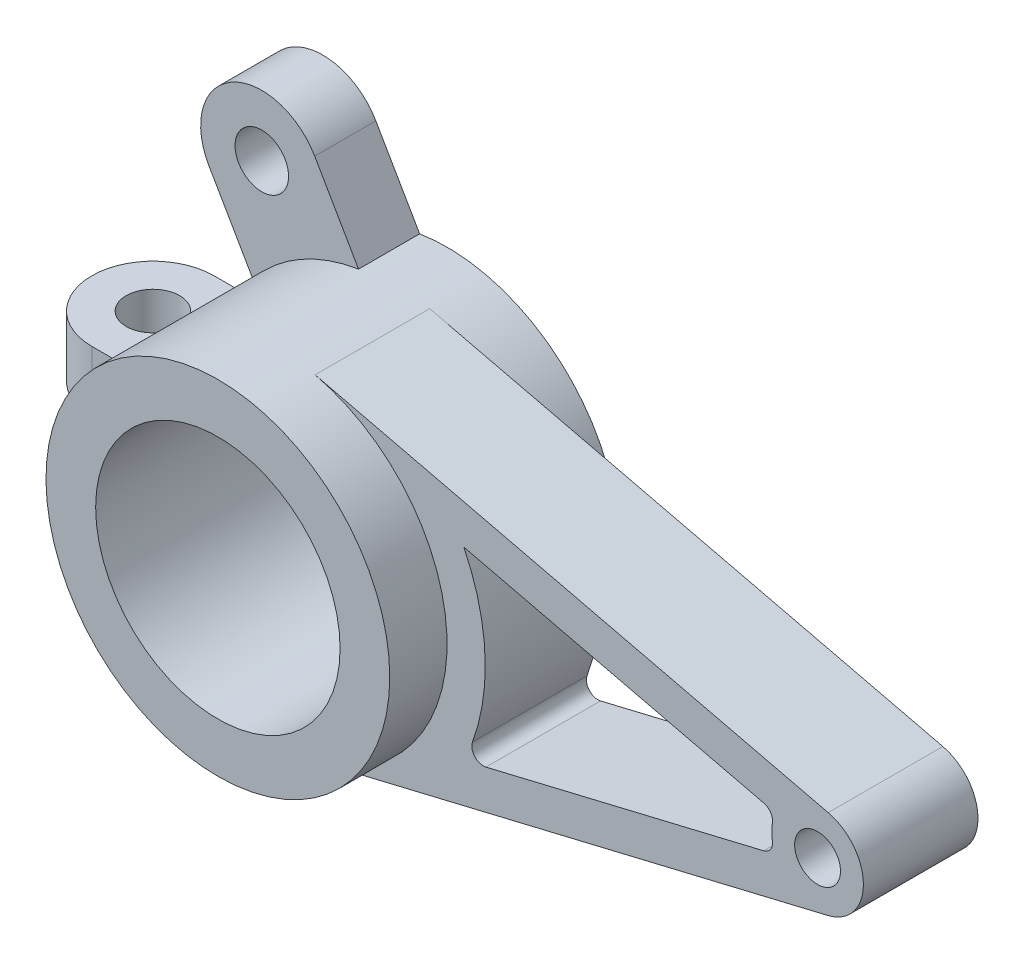
ISO-10303-21;
HEADER;
FILE_DESCRIPTION(('STEP AP214'),'2;1');
FILE_NAME('part.step','',(''),(''),'','','');
FILE_SCHEMA(('AUTOMOTIVE_DESIGN { 1 0 10303 214 1 1 1 1 }'));
ENDSEC;
DATA;
#1=APPLICATION_CONTEXT('core data for automotive mechanical design processes');
#2=APPLICATION_PROTOCOL_DEFINITION('international standard','automotive_design',2000,#1);
#3=PRODUCT_CONTEXT('',#1,'mechanical');
#4=PRODUCT('Part','Part','',(#3));
#5=PRODUCT_RELATED_PRODUCT_CATEGORY('part','',(#4));
#6=PRODUCT_DEFINITION_FORMATION('','',#4);
#7=PRODUCT_DEFINITION_CONTEXT('part definition',#1,'design');
#8=PRODUCT_DEFINITION('design','',#6,#7);
#9=PRODUCT_DEFINITION_SHAPE('','',#8);
#10=(LENGTH_UNIT() NAMED_UNIT(*) SI_UNIT(.MILLI.,.METRE.));
#11=(NAMED_UNIT(*) PLANE_ANGLE_UNIT() SI_UNIT($,.RADIAN.));
#12=(NAMED_UNIT(*) SI_UNIT($,.STERADIAN.) SOLID_ANGLE_UNIT());
#13=UNCERTAINTY_MEASURE_WITH_UNIT(LENGTH_MEASURE(1.E-05),#10,'distance_accuracy_value','');
#14=(GEOMETRIC_REPRESENTATION_CONTEXT(3) GLOBAL_UNCERTAINTY_ASSIGNED_CONTEXT((#13)) GLOBAL_UNIT_ASSIGNED_CONTEXT((#10,
#11,#12)) REPRESENTATION_CONTEXT('',''));
#15=CARTESIAN_POINT('',(0.,0.,0.));
#16=DIRECTION('',(0.,0.,1.));
#17=DIRECTION('',(1.,0.,0.));
#18=AXIS2_PLACEMENT_3D('',#15,#16,#17);
#19=CARTESIAN_POINT('',(0.,0.,60.));
#20=DIRECTION('',(0.,0.,-1.));
#21=DIRECTION('',(-1.,0.,0.));
#22=AXIS2_PLACEMENT_3D('',#19,#20,#21);
#23=CYLINDRICAL_SURFACE('',#22,45.);
#24=DIRECTION('',(0.,0.,-1.));
#25=VECTOR('',#24,1.);
#26=CARTESIAN_POINT('',(10.4577464788732,-43.7679738916895,45.));
#27=LINE('',#26,#25);
#28=CARTESIAN_POINT('',(10.4577464788732,-43.7679738916895,45.));
#29=VERTEX_POINT('',#28);
#30=CARTESIAN_POINT('',(10.4577464788732,-43.7679738916895,15.));
#31=VERTEX_POINT('',#30);
#32=EDGE_CURVE('E369',#29,#31,#27,.T.);
#33=ORIENTED_EDGE('',*,*,#32,.F.);
#34=CARTESIAN_POINT('',(0.,0.,45.));
#35=DIRECTION('',(0.,0.,1.));
#36=DIRECTION('',(1.,0.,0.));
#37=AXIS2_PLACEMENT_3D('',#34,#35,#36);
#38=CIRCLE('',#37,45.);
#39=CARTESIAN_POINT('',(10.4577464788732,43.7679738916895,45.));
#40=VERTEX_POINT('',#39);
#41=EDGE_CURVE('E332',#29,#40,#38,.T.);
#42=ORIENTED_EDGE('',*,*,#41,.T.);
#43=DIRECTION('',(0.,0.,-1.));
#44=VECTOR('',#43,1.);
#45=CARTESIAN_POINT('',(10.4577464788732,43.7679738916895,45.));
#46=LINE('',#45,#44);
#47=CARTESIAN_POINT('',(10.4577464788732,43.7679738916895,15.));
#48=VERTEX_POINT('',#47);
#49=EDGE_CURVE('E373',#40,#48,#46,.T.);
#50=ORIENTED_EDGE('',*,*,#49,.T.);
#51=CARTESIAN_POINT('',(0.,0.,15.));
#52=DIRECTION('',(0.,0.,1.));
#53=DIRECTION('',(1.,0.,0.));
#54=AXIS2_PLACEMENT_3D('',#51,#52,#53);
#55=CIRCLE('',#54,45.);
#56=EDGE_CURVE('E306',#31,#48,#55,.T.);
#57=ORIENTED_EDGE('',*,*,#56,.F.);
#58=EDGE_LOOP('',(#33,#42,#50,#57));
#59=FACE_BOUND('',#58,.T.);
#60=CARTESIAN_POINT('',(0.,0.,60.));
#61=DIRECTION('',(0.,0.,1.));
#62=DIRECTION('',(1.,0.,0.));
#63=AXIS2_PLACEMENT_3D('',#60,#61,#62);
#64=CIRCLE('',#63,45.);
#65=CARTESIAN_POINT('',(45.,0.,60.));
#66=VERTEX_POINT('',#65);
#67=EDGE_CURVE('E49',#66,#66,#64,.T.);
#68=ORIENTED_EDGE('',*,*,#67,.F.);
#69=EDGE_LOOP('',(#68));
#70=FACE_BOUND('',#69,.T.);
#71=CARTESIAN_POINT('',(0.,0.,0.));
#72=DIRECTION('',(0.,0.,1.));
#73=DIRECTION('',(1.,0.,0.));
#74=AXIS2_PLACEMENT_3D('',#71,#72,#73);
#75=CIRCLE('',#74,45.);
#76=CARTESIAN_POINT('',(-34.8861473053641,28.4245796132227,0.));
#77=VERTEX_POINT('',#76);
#78=CARTESIAN_POINT('',(-44.2831796509691,8.,0.));
#79=VERTEX_POINT('',#78);
#80=EDGE_CURVE('E405',#77,#79,#75,.T.);
#81=ORIENTED_EDGE('',*,*,#80,.T.);
#82=DIRECTION('',(0.,0.,-1.));
#83=VECTOR('',#82,1.);
#84=CARTESIAN_POINT('',(-44.2831796509691,8.,60.));
#85=LINE('',#84,#83);
#86=CARTESIAN_POINT('',(-44.2831796509691,8.,32.));
#87=VERTEX_POINT('',#86);
#88=EDGE_CURVE('E60',#79,#87,#85,.F.);
#89=ORIENTED_EDGE('',*,*,#88,.T.);
#90=CARTESIAN_POINT('',(0.,0.,32.));
#91=DIRECTION('',(0.,0.,-1.));
#92=DIRECTION('',(-1.,0.,0.));
#93=AXIS2_PLACEMENT_3D('',#90,#91,#92);
#94=CIRCLE('',#93,45.);
#95=CARTESIAN_POINT('',(-44.2831796509691,-8.,32.));
#96=VERTEX_POINT('',#95);
#97=EDGE_CURVE('E11',#96,#87,#94,.T.);
#98=ORIENTED_EDGE('',*,*,#97,.F.);
#99=DIRECTION('',(0.,0.,-1.));
#100=VECTOR('',#99,1.);
#101=CARTESIAN_POINT('',(-44.2831796509691,-8.,60.));
#102=LINE('',#101,#100);
#103=CARTESIAN_POINT('',(-44.2831796509691,-8.,0.));
#104=VERTEX_POINT('',#103);
#105=EDGE_CURVE('E65',#104,#96,#102,.F.);
#106=ORIENTED_EDGE('',*,*,#105,.F.);
#107=CARTESIAN_POINT('',(-35.9271712475847,-27.0968331387032,0.));
#108=VERTEX_POINT('',#107);
#109=EDGE_CURVE('E401',#104,#108,#75,.T.);
#110=ORIENTED_EDGE('',*,*,#109,.T.);
#111=DIRECTION('',(0.,0.,-1.));
#112=VECTOR('',#111,1.);
#113=CARTESIAN_POINT('',(-35.9271712475847,-27.0968331387032,16.));
#114=LINE('',#113,#112);
#115=CARTESIAN_POINT('',(-35.9271712475847,-27.0968331387032,16.));
#116=VERTEX_POINT('',#115);
#117=EDGE_CURVE('E263',#116,#108,#114,.T.);
#118=ORIENTED_EDGE('',*,*,#117,.F.);
#119=CARTESIAN_POINT('',(0.,0.,16.));
#120=DIRECTION('',(0.,0.,1.));
#121=DIRECTION('',(1.,0.,0.));
#122=AXIS2_PLACEMENT_3D('',#119,#120,#121);
#123=CIRCLE('',#122,45.);
#124=CARTESIAN_POINT('',(-8.83362462507804,-44.1244498660688,16.));
#125=VERTEX_POINT('',#124);
#126=EDGE_CURVE('E234',#116,#125,#123,.T.);
#127=ORIENTED_EDGE('',*,*,#126,.T.);
#128=DIRECTION('',(0.,0.,-1.));
#129=VECTOR('',#128,1.);
#130=CARTESIAN_POINT('',(-8.83362462507804,-44.1244498660688,16.));
#131=LINE('',#130,#129);
#132=CARTESIAN_POINT('',(-8.83362462507804,-44.1244498660688,0.));
#133=VERTEX_POINT('',#132);
#134=EDGE_CURVE('E250',#125,#133,#131,.T.);
#135=ORIENTED_EDGE('',*,*,#134,.T.);
#136=CARTESIAN_POINT('',(-7.17333438426207,44.4245796132227,0.));
#137=VERTEX_POINT('',#136);
#138=EDGE_CURVE('E397',#133,#137,#75,.T.);
#139=ORIENTED_EDGE('',*,*,#138,.T.);
#140=DIRECTION('',(0.,0.,-1.));
#141=VECTOR('',#140,1.);
#142=CARTESIAN_POINT('',(-7.17333438426207,44.4245796132227,16.));
#143=LINE('',#142,#141);
#144=CARTESIAN_POINT('',(-7.17333438426207,44.4245796132227,16.));
#145=VERTEX_POINT('',#144);
#146=EDGE_CURVE('E296',#145,#137,#143,.T.);
#147=ORIENTED_EDGE('',*,*,#146,.F.);
#148=CARTESIAN_POINT('',(0.,0.,16.));
#149=DIRECTION('',(0.,0.,-1.));
#150=DIRECTION('',(1.,0.,0.));
#151=AXIS2_PLACEMENT_3D('',#148,#149,#150);
#152=CIRCLE('',#151,45.);
#153=CARTESIAN_POINT('',(-34.8861473053641,28.4245796132227,16.));
#154=VERTEX_POINT('',#153);
#155=EDGE_CURVE('E274',#154,#145,#152,.T.);
#156=ORIENTED_EDGE('',*,*,#155,.F.);
#157=DIRECTION('',(0.,0.,-1.));
#158=VECTOR('',#157,1.);
#159=CARTESIAN_POINT('',(-34.8861473053641,28.4245796132227,16.));
#160=LINE('',#159,#158);
#161=EDGE_CURVE('E285',#154,#77,#160,.T.);
#162=ORIENTED_EDGE('',*,*,#161,.T.);
#163=EDGE_LOOP('',(#81,#89,#98,#106,#110,#118,#127,#135,#139,#147,#156,#162));
#164=FACE_BOUND('',#163,.T.);
#165=ADVANCED_FACE('F43',(#59,#70,#164),#23,.T.);
#166=CARTESIAN_POINT('',(0.,0.,60.));
#167=DIRECTION('',(0.,0.,1.));
#168=DIRECTION('',(1.,0.,0.));
#169=AXIS2_PLACEMENT_3D('',#166,#167,#168);
#170=PLANE('',#169);
#171=ORIENTED_EDGE('',*,*,#67,.T.);
#172=EDGE_LOOP('',(#171));
#173=FACE_BOUND('',#172,.T.);
#174=CARTESIAN_POINT('',(0.,0.,60.));
#175=DIRECTION('',(0.,0.,1.));
#176=DIRECTION('',(1.,0.,0.));
#177=AXIS2_PLACEMENT_3D('',#174,#175,#176);
#178=CIRCLE('',#177,32.);
#179=CARTESIAN_POINT('',(32.,0.,60.));
#180=VERTEX_POINT('',#179);
#181=EDGE_CURVE('E395',#180,#180,#178,.T.);
#182=ORIENTED_EDGE('',*,*,#181,.F.);
#183=EDGE_LOOP('',(#182));
#184=FACE_BOUND('',#183,.T.);
#185=ADVANCED_FACE('F432',(#173,#184),#170,.T.);
#186=CARTESIAN_POINT('',(0.,0.,0.));
#187=DIRECTION('',(0.,0.,1.));
#188=DIRECTION('',(1.,0.,0.));
#189=AXIS2_PLACEMENT_3D('',#186,#187,#188);
#190=PLANE('',#189);
#191=ORIENTED_EDGE('',*,*,#109,.F.);
#192=DIRECTION('',(-1.,0.,0.));
#193=VECTOR('',#192,1.);
#194=CARTESIAN_POINT('',(-61.,-8.,0.));
#195=LINE('',#194,#193);
#196=CARTESIAN_POINT('',(-61.,-8.,0.));
#197=VERTEX_POINT('',#196);
#198=EDGE_CURVE('E208',#104,#197,#195,.T.);
#199=ORIENTED_EDGE('',*,*,#198,.T.);
#200=DIRECTION('',(0.,-1.,0.));
#201=VECTOR('',#200,1.);
#202=CARTESIAN_POINT('',(-61.,8.,0.));
#203=LINE('',#202,#201);
#204=CARTESIAN_POINT('',(-61.,8.,0.));
#205=VERTEX_POINT('',#204);
#206=EDGE_CURVE('E207',#205,#197,#203,.T.);
#207=ORIENTED_EDGE('',*,*,#206,.F.);
#208=DIRECTION('',(-1.,0.,0.));
#209=VECTOR('',#208,1.);
#210=CARTESIAN_POINT('',(-45.,8.,0.));
#211=LINE('',#210,#209);
#212=EDGE_CURVE('E191',#79,#205,#211,.T.);
#213=ORIENTED_EDGE('',*,*,#212,.F.);
#214=ORIENTED_EDGE('',*,*,#80,.F.);
#215=DIRECTION('',(0.5,-0.866025403784439,0.));
#216=VECTOR('',#215,1.);
#217=CARTESIAN_POINT('',(-34.8861473053641,28.4245796132227,0.));
#218=LINE('',#217,#216);
#219=CARTESIAN_POINT('',(-46.356406460551,48.2916512459885,0.));
#220=VERTEX_POINT('',#219);
#221=EDGE_CURVE('E279',#220,#77,#218,.T.);
#222=ORIENTED_EDGE('',*,*,#221,.F.);
#223=CARTESIAN_POINT('',(-32.5000000000001,56.2916512459885,0.));
#224=DIRECTION('',(0.,0.,1.));
#225=DIRECTION('',(1.,0.,0.));
#226=AXIS2_PLACEMENT_3D('',#223,#224,#225);
#227=CIRCLE('',#226,16.);
#228=CARTESIAN_POINT('',(-18.6435935394491,64.2916512459885,0.));
#229=VERTEX_POINT('',#228);
#230=EDGE_CURVE('E289',#229,#220,#227,.T.);
#231=ORIENTED_EDGE('',*,*,#230,.F.);
#232=DIRECTION('',(-0.5,0.866025403784439,0.));
#233=VECTOR('',#232,1.);
#234=CARTESIAN_POINT('',(-7.17333438426207,44.4245796132227,0.));
#235=LINE('',#234,#233);
#236=EDGE_CURVE('E272',#137,#229,#235,.T.);
#237=ORIENTED_EDGE('',*,*,#236,.F.);
#238=ORIENTED_EDGE('',*,*,#138,.F.);
#239=DIRECTION('',(-0.532113022730173,-0.846673331953333,0.));
#240=VECTOR('',#239,1.);
#241=CARTESIAN_POINT('',(13.5467733112533,-8.51380836368278,0.));
#242=LINE('',#241,#240);
#243=CARTESIAN_POINT('',(-21.0405731662079,-63.5475749406494,0.));
#244=VERTEX_POINT('',#243);
#245=EDGE_CURVE('E255',#133,#244,#242,.T.);
#246=ORIENTED_EDGE('',*,*,#245,.T.);
#247=CARTESIAN_POINT('',(-34.5873464774612,-55.0337665769666,0.));
#248=DIRECTION('',(0.,0.,1.));
#249=DIRECTION('',(1.,0.,0.));
#250=AXIS2_PLACEMENT_3D('',#247,#248,#249);
#251=CIRCLE('',#250,16.);
#252=CARTESIAN_POINT('',(-48.1341197887146,-46.5199582132839,0.));
#253=VERTEX_POINT('',#252);
#254=EDGE_CURVE('E248',#253,#244,#251,.T.);
#255=ORIENTED_EDGE('',*,*,#254,.F.);
#256=DIRECTION('',(-0.532113022730173,-0.846673331953333,0.));
#257=VECTOR('',#256,1.);
#258=CARTESIAN_POINT('',(-13.5467733112533,8.51380836368277,0.));
#259=LINE('',#258,#257);
#260=EDGE_CURVE('E231',#108,#253,#259,.T.);
#261=ORIENTED_EDGE('',*,*,#260,.F.);
#262=EDGE_LOOP('',(#191,#199,#207,#213,#214,#222,#231,#237,#238,#246,#255,#261));
#263=FACE_BOUND('',#262,.T.);
#264=CARTESIAN_POINT('',(0.,0.,0.));
#265=DIRECTION('',(0.,0.,1.));
#266=DIRECTION('',(1.,0.,0.));
#267=AXIS2_PLACEMENT_3D('',#264,#265,#266);
#268=CIRCLE('',#267,32.);
#269=CARTESIAN_POINT('',(32.,0.,0.));
#270=VERTEX_POINT('',#269);
#271=EDGE_CURVE('E382',#270,#270,#268,.T.);
#272=ORIENTED_EDGE('',*,*,#271,.T.);
#273=EDGE_LOOP('',(#272));
#274=FACE_BOUND('',#273,.T.);
#275=CARTESIAN_POINT('',(-32.5000000000001,56.2916512459885,0.));
#276=DIRECTION('',(0.,0.,1.));
#277=DIRECTION('',(1.,0.,0.));
#278=AXIS2_PLACEMENT_3D('',#275,#276,#277);
#279=CIRCLE('',#278,7.);
#280=CARTESIAN_POINT('',(-25.5000000000001,56.2916512459885,0.));
#281=VERTEX_POINT('',#280);
#282=EDGE_CURVE('E269',#281,#281,#279,.T.);
#283=ORIENTED_EDGE('',*,*,#282,.T.);
#284=EDGE_LOOP('',(#283));
#285=FACE_BOUND('',#284,.T.);
#286=CARTESIAN_POINT('',(-34.5873464774612,-55.0337665769666,0.));
#287=DIRECTION('',(0.,0.,1.));
#288=DIRECTION('',(1.,0.,0.));
#289=AXIS2_PLACEMENT_3D('',#286,#287,#288);
#290=CIRCLE('',#289,7.);
#291=CARTESIAN_POINT('',(-27.5873464774612,-55.0337665769666,0.));
#292=VERTEX_POINT('',#291);
#293=EDGE_CURVE('E240',#292,#292,#290,.T.);
#294=ORIENTED_EDGE('',*,*,#293,.T.);
#295=EDGE_LOOP('',(#294));
#296=FACE_BOUND('',#295,.T.);
#297=ADVANCED_FACE('F210',(#263,#274,#285,#296),#190,.F.);
#298=CARTESIAN_POINT('',(0.,0.,60.));
#299=DIRECTION('',(0.,0.,-1.));
#300=DIRECTION('',(-1.,0.,0.));
#301=AXIS2_PLACEMENT_3D('',#298,#299,#300);
#302=CYLINDRICAL_SURFACE('',#301,32.);
#303=ORIENTED_EDGE('',*,*,#181,.T.);
#304=EDGE_LOOP('',(#303));
#305=FACE_BOUND('',#304,.T.);
#306=ORIENTED_EDGE('',*,*,#271,.F.);
#307=EDGE_LOOP('',(#306));
#308=FACE_BOUND('',#307,.T.);
#309=ADVANCED_FACE('F446',(#305,#308),#302,.F.);
#310=CARTESIAN_POINT('',(10.4577464788732,-43.7679738916895,45.));
#311=DIRECTION('',(-0.232394366197183,0.972621642037545,0.));
#312=DIRECTION('',(-0.972621642037545,-0.232394366197183,0.));
#313=AXIS2_PLACEMENT_3D('',#310,#311,#312);
#314=PLANE('',#313);
#315=DIRECTION('',(0.972621642037545,0.232394366197183,0.));
#316=VECTOR('',#315,1.);
#317=CARTESIAN_POINT('',(10.4577464788732,-43.7679738916895,15.));
#318=LINE('',#317,#316);
#319=CARTESIAN_POINT('',(144.788732394366,-11.6714597044506,15.));
#320=VERTEX_POINT('',#319);
#321=EDGE_CURVE('E360',#31,#320,#318,.T.);
#322=ORIENTED_EDGE('',*,*,#321,.T.);
#323=DIRECTION('',(0.,0.,-1.));
#324=VECTOR('',#323,1.);
#325=CARTESIAN_POINT('',(144.788732394366,-11.6714597044506,45.));
#326=LINE('',#325,#324);
#327=CARTESIAN_POINT('',(144.788732394366,-11.6714597044506,45.));
#328=VERTEX_POINT('',#327);
#329=EDGE_CURVE('E377',#328,#320,#326,.T.);
#330=ORIENTED_EDGE('',*,*,#329,.F.);
#331=DIRECTION('',(0.972621642037545,0.232394366197183,0.));
#332=VECTOR('',#331,1.);
#333=CARTESIAN_POINT('',(10.4577464788732,-43.7679738916895,45.));
#334=LINE('',#333,#332);
#335=EDGE_CURVE('E323',#29,#328,#334,.T.);
#336=ORIENTED_EDGE('',*,*,#335,.F.);
#337=ORIENTED_EDGE('',*,*,#32,.T.);
#338=EDGE_LOOP('',(#322,#330,#336,#337));
#339=FACE_BOUND('',#338,.T.);
#340=ADVANCED_FACE('F455',(#339),#314,.F.);
#341=CARTESIAN_POINT('',(142.,0.,45.));
#342=DIRECTION('',(0.,0.,-1.));
#343=DIRECTION('',(-1.,0.,0.));
#344=AXIS2_PLACEMENT_3D('',#341,#342,#343);
#345=CYLINDRICAL_SURFACE('',#344,12.);
#346=CARTESIAN_POINT('',(142.,0.,15.));
#347=DIRECTION('',(0.,0.,1.));
#348=DIRECTION('',(1.,0.,0.));
#349=AXIS2_PLACEMENT_3D('',#346,#347,#348);
#350=CIRCLE('',#349,12.);
#351=CARTESIAN_POINT('',(144.788732394366,11.6714597044505,15.));
#352=VERTEX_POINT('',#351);
#353=EDGE_CURVE('E365',#320,#352,#350,.T.);
#354=ORIENTED_EDGE('',*,*,#353,.T.);
#355=DIRECTION('',(0.,0.,-1.));
#356=VECTOR('',#355,1.);
#357=CARTESIAN_POINT('',(144.788732394366,11.6714597044505,45.));
#358=LINE('',#357,#356);
#359=CARTESIAN_POINT('',(144.788732394366,11.6714597044505,45.));
#360=VERTEX_POINT('',#359);
#361=EDGE_CURVE('E376',#360,#352,#358,.T.);
#362=ORIENTED_EDGE('',*,*,#361,.F.);
#363=CARTESIAN_POINT('',(142.,0.,45.));
#364=DIRECTION('',(0.,0.,1.));
#365=DIRECTION('',(1.,0.,0.));
#366=AXIS2_PLACEMENT_3D('',#363,#364,#365);
#367=CIRCLE('',#366,12.);
#368=EDGE_CURVE('E329',#328,#360,#367,.T.);
#369=ORIENTED_EDGE('',*,*,#368,.F.);
#370=ORIENTED_EDGE('',*,*,#329,.T.);
#371=EDGE_LOOP('',(#354,#362,#369,#370));
#372=FACE_BOUND('',#371,.T.);
#373=ADVANCED_FACE('F506',(#372),#345,.T.);
#374=CARTESIAN_POINT('',(10.4577464788732,43.7679738916895,45.));
#375=DIRECTION('',(0.232394366197183,0.972621642037545,0.));
#376=DIRECTION('',(-0.972621642037545,0.232394366197183,0.));
#377=AXIS2_PLACEMENT_3D('',#374,#375,#376);
#378=PLANE('',#377);
#379=DIRECTION('',(0.972621642037545,-0.232394366197183,0.));
#380=VECTOR('',#379,1.);
#381=CARTESIAN_POINT('',(10.4577464788732,43.7679738916895,15.));
#382=LINE('',#381,#380);
#383=EDGE_CURVE('E362',#48,#352,#382,.T.);
#384=ORIENTED_EDGE('',*,*,#383,.F.);
#385=ORIENTED_EDGE('',*,*,#49,.F.);
#386=DIRECTION('',(0.972621642037545,-0.232394366197183,0.));
#387=VECTOR('',#386,1.);
#388=CARTESIAN_POINT('',(10.4577464788732,43.7679738916895,45.));
#389=LINE('',#388,#387);
#390=EDGE_CURVE('E330',#40,#360,#389,.T.);
#391=ORIENTED_EDGE('',*,*,#390,.T.);
#392=ORIENTED_EDGE('',*,*,#361,.T.);
#393=EDGE_LOOP('',(#384,#385,#391,#392));
#394=FACE_BOUND('',#393,.T.);
#395=ADVANCED_FACE('F505',(#394),#378,.T.);
#396=CARTESIAN_POINT('',(127.210737827939,-2.50553874566784,45.));
#397=DIRECTION('',(0.,0.,-1.));
#398=DIRECTION('',(-1.,0.,0.));
#399=AXIS2_PLACEMENT_3D('',#396,#397,#398);
#400=CYLINDRICAL_SURFACE('',#399,2.99999999999999);
#401=CARTESIAN_POINT('',(127.210737827939,-2.50553874566784,15.));
#402=DIRECTION('',(0.,0.,1.));
#403=DIRECTION('',(1.,0.,0.));
#404=AXIS2_PLACEMENT_3D('',#401,#402,#403);
#405=CIRCLE('',#404,2.99999999999999);
#406=CARTESIAN_POINT('',(127.90792092653,-5.42340367178045,15.));
#407=VERTEX_POINT('',#406);
#408=CARTESIAN_POINT('',(130.168590262351,-2.00443099653427,15.));
#409=VERTEX_POINT('',#408);
#410=EDGE_CURVE('E336',#407,#409,#405,.T.);
#411=ORIENTED_EDGE('',*,*,#410,.F.);
#412=DIRECTION('',(0.,0.,-1.));
#413=VECTOR('',#412,1.);
#414=CARTESIAN_POINT('',(127.90792092653,-5.42340367178045,45.));
#415=LINE('',#414,#413);
#416=CARTESIAN_POINT('',(127.90792092653,-5.42340367178045,45.));
#417=VERTEX_POINT('',#416);
#418=EDGE_CURVE('E372',#417,#407,#415,.T.);
#419=ORIENTED_EDGE('',*,*,#418,.F.);
#420=CARTESIAN_POINT('',(127.210737827939,-2.50553874566784,45.));
#421=DIRECTION('',(0.,0.,1.));
#422=DIRECTION('',(1.,0.,0.));
#423=AXIS2_PLACEMENT_3D('',#420,#421,#422);
#424=CIRCLE('',#423,2.99999999999999);
#425=CARTESIAN_POINT('',(130.168590262351,-2.00443099653427,45.));
#426=VERTEX_POINT('',#425);
#427=EDGE_CURVE('E304',#417,#426,#424,.T.);
#428=ORIENTED_EDGE('',*,*,#427,.T.);
#429=DIRECTION('',(0.,0.,-1.));
#430=VECTOR('',#429,1.);
#431=CARTESIAN_POINT('',(130.168590262351,-2.00443099653427,45.));
#432=LINE('',#431,#430);
#433=EDGE_CURVE('E331',#426,#409,#432,.T.);
#434=ORIENTED_EDGE('',*,*,#433,.T.);
#435=EDGE_LOOP('',(#411,#419,#428,#434));
#436=FACE_BOUND('',#435,.T.);
#437=ADVANCED_FACE('F504',(#436),#400,.F.);
#438=CARTESIAN_POINT('',(8.13380281690141,-34.0417574713141,45.));
#439=DIRECTION('',(-0.232394366197183,0.972621642037545,0.));
#440=DIRECTION('',(-0.972621642037545,-0.232394366197183,0.));
#441=AXIS2_PLACEMENT_3D('',#438,#439,#440);
#442=PLANE('',#441);
#443=DIRECTION('',(0.972621642037545,0.232394366197183,0.));
#444=VECTOR('',#443,1.);
#445=CARTESIAN_POINT('',(8.13380281690141,-34.0417574713141,15.));
#446=LINE('',#445,#444);
#447=CARTESIAN_POINT('',(55.1829610349817,-22.800017794109,15.));
#448=VERTEX_POINT('',#447);
#449=EDGE_CURVE('E342',#448,#407,#446,.T.);
#450=ORIENTED_EDGE('',*,*,#449,.F.);
#451=DIRECTION('',(0.,0.,-1.));
#452=VECTOR('',#451,1.);
#453=CARTESIAN_POINT('',(55.1829610349817,-22.800017794109,45.));
#454=LINE('',#453,#452);
#455=CARTESIAN_POINT('',(55.1829610349817,-22.800017794109,45.));
#456=VERTEX_POINT('',#455);
#457=EDGE_CURVE('E392',#456,#448,#454,.T.);
#458=ORIENTED_EDGE('',*,*,#457,.F.);
#459=DIRECTION('',(0.972621642037545,0.232394366197183,0.));
#460=VECTOR('',#459,1.);
#461=CARTESIAN_POINT('',(8.13380281690141,-34.0417574713141,45.));
#462=LINE('',#461,#460);
#463=EDGE_CURVE('E307',#456,#417,#462,.T.);
#464=ORIENTED_EDGE('',*,*,#463,.T.);
#465=ORIENTED_EDGE('',*,*,#418,.T.);
#466=EDGE_LOOP('',(#450,#458,#464,#465));
#467=FACE_BOUND('',#466,.T.);
#468=ADVANCED_FACE('F531',(#467),#442,.T.);
#469=CARTESIAN_POINT('',(54.4857779363902,-19.8821528679964,45.));
#470=DIRECTION('',(0.,0.,-1.));
#471=DIRECTION('',(-1.,0.,0.));
#472=AXIS2_PLACEMENT_3D('',#469,#470,#471);
#473=CYLINDRICAL_SURFACE('',#472,3.00000000000001);
#474=CARTESIAN_POINT('',(54.4857779363902,-19.8821528679964,15.));
#475=DIRECTION('',(0.,0.,1.));
#476=DIRECTION('',(1.,0.,0.));
#477=AXIS2_PLACEMENT_3D('',#474,#475,#476);
#478=CIRCLE('',#477,3.00000000000001);
#479=CARTESIAN_POINT('',(51.6675480431286,-18.8537656506862,15.));
#480=VERTEX_POINT('',#479);
#481=EDGE_CURVE('E341',#480,#448,#478,.T.);
#482=ORIENTED_EDGE('',*,*,#481,.F.);
#483=DIRECTION('',(0.,0.,-1.));
#484=VECTOR('',#483,1.);
#485=CARTESIAN_POINT('',(51.6675480431286,-18.8537656506862,45.));
#486=LINE('',#485,#484);
#487=CARTESIAN_POINT('',(51.6675480431286,-18.8537656506862,45.));
#488=VERTEX_POINT('',#487);
#489=EDGE_CURVE('E388',#488,#480,#486,.T.);
#490=ORIENTED_EDGE('',*,*,#489,.F.);
#491=CARTESIAN_POINT('',(54.4857779363902,-19.8821528679964,45.));
#492=DIRECTION('',(0.,0.,1.));
#493=DIRECTION('',(1.,0.,0.));
#494=AXIS2_PLACEMENT_3D('',#491,#492,#493);
#495=CIRCLE('',#494,3.00000000000001);
#496=EDGE_CURVE('E315',#488,#456,#495,.T.);
#497=ORIENTED_EDGE('',*,*,#496,.T.);
#498=ORIENTED_EDGE('',*,*,#457,.T.);
#499=EDGE_LOOP('',(#482,#490,#497,#498));
#500=FACE_BOUND('',#499,.T.);
#501=ADVANCED_FACE('F530',(#500),#473,.F.);
#502=CARTESIAN_POINT('',(0.,0.,45.));
#503=DIRECTION('',(0.,0.,-1.));
#504=DIRECTION('',(-1.,0.,0.));
#505=AXIS2_PLACEMENT_3D('',#502,#503,#504);
#506=CYLINDRICAL_SURFACE('',#505,55.);
#507=CARTESIAN_POINT('',(0.,0.,15.));
#508=DIRECTION('',(0.,0.,1.));
#509=DIRECTION('',(1.,0.,0.));
#510=AXIS2_PLACEMENT_3D('',#507,#508,#509);
#511=CIRCLE('',#510,55.);
#512=CARTESIAN_POINT('',(49.398644333714,24.1820995364594,15.));
#513=VERTEX_POINT('',#512);
#514=EDGE_CURVE('E347',#480,#513,#511,.T.);
#515=ORIENTED_EDGE('',*,*,#514,.T.);
#516=DIRECTION('',(0.,0.,-1.));
#517=VECTOR('',#516,1.);
#518=CARTESIAN_POINT('',(49.398644333714,24.1820995364594,45.));
#519=LINE('',#518,#517);
#520=CARTESIAN_POINT('',(49.398644333714,24.1820995364594,45.));
#521=VERTEX_POINT('',#520);
#522=EDGE_CURVE('E390',#521,#513,#519,.T.);
#523=ORIENTED_EDGE('',*,*,#522,.F.);
#524=CARTESIAN_POINT('',(0.,0.,45.));
#525=DIRECTION('',(0.,0.,1.));
#526=DIRECTION('',(1.,0.,0.));
#527=AXIS2_PLACEMENT_3D('',#524,#525,#526);
#528=CIRCLE('',#527,55.);
#529=EDGE_CURVE('E314',#488,#521,#528,.T.);
#530=ORIENTED_EDGE('',*,*,#529,.F.);
#531=ORIENTED_EDGE('',*,*,#489,.T.);
#532=EDGE_LOOP('',(#515,#523,#530,#531));
#533=FACE_BOUND('',#532,.T.);
#534=ADVANCED_FACE('F525',(#533),#506,.T.);
#535=CARTESIAN_POINT('',(8.1338028169014,34.041757471314,45.));
#536=DIRECTION('',(0.232394366197183,0.972621642037545,0.));
#537=DIRECTION('',(-0.972621642037545,0.232394366197183,0.));
#538=AXIS2_PLACEMENT_3D('',#535,#536,#537);
#539=PLANE('',#538);
#540=DIRECTION('',(0.972621642037545,-0.232394366197183,0.));
#541=VECTOR('',#540,1.);
#542=CARTESIAN_POINT('',(8.1338028169014,34.041757471314,15.));
#543=LINE('',#542,#541);
#544=CARTESIAN_POINT('',(127.90792092653,5.42340367178043,15.));
#545=VERTEX_POINT('',#544);
#546=EDGE_CURVE('E350',#513,#545,#543,.T.);
#547=ORIENTED_EDGE('',*,*,#546,.T.);
#548=DIRECTION('',(0.,0.,-1.));
#549=VECTOR('',#548,1.);
#550=CARTESIAN_POINT('',(127.90792092653,5.42340367178043,45.));
#551=LINE('',#550,#549);
#552=CARTESIAN_POINT('',(127.90792092653,5.42340367178043,45.));
#553=VERTEX_POINT('',#552);
#554=EDGE_CURVE('E383',#553,#545,#551,.T.);
#555=ORIENTED_EDGE('',*,*,#554,.F.);
#556=DIRECTION('',(0.972621642037545,-0.232394366197183,0.));
#557=VECTOR('',#556,1.);
#558=CARTESIAN_POINT('',(8.1338028169014,34.041757471314,45.));
#559=LINE('',#558,#557);
#560=EDGE_CURVE('E319',#521,#553,#559,.T.);
#561=ORIENTED_EDGE('',*,*,#560,.F.);
#562=ORIENTED_EDGE('',*,*,#522,.T.);
#563=EDGE_LOOP('',(#547,#555,#561,#562));
#564=FACE_BOUND('',#563,.T.);
#565=ADVANCED_FACE('F521',(#564),#539,.F.);
#566=CARTESIAN_POINT('',(127.210737827939,2.50553874566781,45.));
#567=DIRECTION('',(0.,0.,-1.));
#568=DIRECTION('',(-1.,0.,0.));
#569=AXIS2_PLACEMENT_3D('',#566,#567,#568);
#570=CYLINDRICAL_SURFACE('',#569,2.99999999999999);
#571=CARTESIAN_POINT('',(127.210737827939,2.50553874566781,15.));
#572=DIRECTION('',(0.,0.,1.));
#573=DIRECTION('',(1.,0.,0.));
#574=AXIS2_PLACEMENT_3D('',#571,#572,#573);
#575=CIRCLE('',#574,2.99999999999999);
#576=CARTESIAN_POINT('',(130.168590262351,2.00443099653425,15.));
#577=VERTEX_POINT('',#576);
#578=EDGE_CURVE('E352',#577,#545,#575,.T.);
#579=ORIENTED_EDGE('',*,*,#578,.F.);
#580=DIRECTION('',(0.,0.,-1.));
#581=VECTOR('',#580,1.);
#582=CARTESIAN_POINT('',(130.168590262351,2.00443099653425,45.));
#583=LINE('',#582,#581);
#584=CARTESIAN_POINT('',(130.168590262351,2.00443099653425,45.));
#585=VERTEX_POINT('',#584);
#586=EDGE_CURVE('E384',#585,#577,#583,.T.);
#587=ORIENTED_EDGE('',*,*,#586,.F.);
#588=CARTESIAN_POINT('',(127.210737827939,2.50553874566781,45.));
#589=DIRECTION('',(0.,0.,1.));
#590=DIRECTION('',(1.,0.,0.));
#591=AXIS2_PLACEMENT_3D('',#588,#589,#590);
#592=CIRCLE('',#591,2.99999999999999);
#593=EDGE_CURVE('E318',#585,#553,#592,.T.);
#594=ORIENTED_EDGE('',*,*,#593,.T.);
#595=ORIENTED_EDGE('',*,*,#554,.T.);
#596=EDGE_LOOP('',(#579,#587,#594,#595));
#597=FACE_BOUND('',#596,.T.);
#598=ADVANCED_FACE('F520',(#597),#570,.F.);
#599=CARTESIAN_POINT('',(142.,0.,45.));
#600=DIRECTION('',(0.,0.,-1.));
#601=DIRECTION('',(-1.,0.,0.));
#602=AXIS2_PLACEMENT_3D('',#599,#600,#601);
#603=CYLINDRICAL_SURFACE('',#602,12.);
#604=CARTESIAN_POINT('',(142.,0.,15.));
#605=DIRECTION('',(0.,0.,1.));
#606=DIRECTION('',(1.,0.,0.));
#607=AXIS2_PLACEMENT_3D('',#604,#605,#606);
#608=CIRCLE('',#607,12.);
#609=EDGE_CURVE('E358',#577,#409,#608,.T.);
#610=ORIENTED_EDGE('',*,*,#609,.T.);
#611=ORIENTED_EDGE('',*,*,#433,.F.);
#612=CARTESIAN_POINT('',(142.,0.,45.));
#613=DIRECTION('',(0.,0.,1.));
#614=DIRECTION('',(1.,0.,0.));
#615=AXIS2_PLACEMENT_3D('',#612,#613,#614);
#616=CIRCLE('',#615,12.);
#617=EDGE_CURVE('E324',#585,#426,#616,.T.);
#618=ORIENTED_EDGE('',*,*,#617,.F.);
#619=ORIENTED_EDGE('',*,*,#586,.T.);
#620=EDGE_LOOP('',(#610,#611,#618,#619));
#621=FACE_BOUND('',#620,.T.);
#622=ADVANCED_FACE('F511',(#621),#603,.T.);
#623=CARTESIAN_POINT('',(142.,0.,45.));
#624=DIRECTION('',(0.,0.,-1.));
#625=DIRECTION('',(-1.,0.,0.));
#626=AXIS2_PLACEMENT_3D('',#623,#624,#625);
#627=CYLINDRICAL_SURFACE('',#626,6.00000000000002);
#628=CARTESIAN_POINT('',(142.,0.,45.));
#629=DIRECTION('',(0.,0.,1.));
#630=DIRECTION('',(1.,0.,0.));
#631=AXIS2_PLACEMENT_3D('',#628,#629,#630);
#632=CIRCLE('',#631,6.00000000000002);
#633=CARTESIAN_POINT('',(148.,0.,45.));
#634=VERTEX_POINT('',#633);
#635=EDGE_CURVE('E305',#634,#634,#632,.T.);
#636=ORIENTED_EDGE('',*,*,#635,.T.);
#637=EDGE_LOOP('',(#636));
#638=FACE_BOUND('',#637,.T.);
#639=CARTESIAN_POINT('',(142.,0.,15.));
#640=DIRECTION('',(0.,0.,1.));
#641=DIRECTION('',(1.,0.,0.));
#642=AXIS2_PLACEMENT_3D('',#639,#640,#641);
#643=CIRCLE('',#642,6.00000000000002);
#644=CARTESIAN_POINT('',(148.,0.,15.));
#645=VERTEX_POINT('',#644);
#646=EDGE_CURVE('E301',#645,#645,#643,.T.);
#647=ORIENTED_EDGE('',*,*,#646,.F.);
#648=EDGE_LOOP('',(#647));
#649=FACE_BOUND('',#648,.T.);
#650=ADVANCED_FACE('F500',(#638,#649),#627,.F.);
#651=CARTESIAN_POINT('',(0.,0.,45.));
#652=DIRECTION('',(0.,0.,1.));
#653=DIRECTION('',(1.,0.,0.));
#654=AXIS2_PLACEMENT_3D('',#651,#652,#653);
#655=PLANE('',#654);
#656=ORIENTED_EDGE('',*,*,#635,.F.);
#657=EDGE_LOOP('',(#656));
#658=FACE_BOUND('',#657,.T.);
#659=ORIENTED_EDGE('',*,*,#427,.F.);
#660=ORIENTED_EDGE('',*,*,#463,.F.);
#661=ORIENTED_EDGE('',*,*,#496,.F.);
#662=ORIENTED_EDGE('',*,*,#529,.T.);
#663=ORIENTED_EDGE('',*,*,#560,.T.);
#664=ORIENTED_EDGE('',*,*,#593,.F.);
#665=ORIENTED_EDGE('',*,*,#617,.T.);
#666=EDGE_LOOP('',(#659,#660,#661,#662,#663,#664,#665));
#667=FACE_BOUND('',#666,.T.);
#668=ORIENTED_EDGE('',*,*,#335,.T.);
#669=ORIENTED_EDGE('',*,*,#368,.T.);
#670=ORIENTED_EDGE('',*,*,#390,.F.);
#671=ORIENTED_EDGE('',*,*,#41,.F.);
#672=EDGE_LOOP('',(#668,#669,#670,#671));
#673=FACE_BOUND('',#672,.T.);
#674=ADVANCED_FACE('F493',(#658,#667,#673),#655,.T.);
#675=CARTESIAN_POINT('',(0.,0.,15.));
#676=DIRECTION('',(0.,0.,1.));
#677=DIRECTION('',(1.,0.,0.));
#678=AXIS2_PLACEMENT_3D('',#675,#676,#677);
#679=PLANE('',#678);
#680=ORIENTED_EDGE('',*,*,#646,.T.);
#681=EDGE_LOOP('',(#680));
#682=FACE_BOUND('',#681,.T.);
#683=ORIENTED_EDGE('',*,*,#410,.T.);
#684=ORIENTED_EDGE('',*,*,#609,.F.);
#685=ORIENTED_EDGE('',*,*,#578,.T.);
#686=ORIENTED_EDGE('',*,*,#546,.F.);
#687=ORIENTED_EDGE('',*,*,#514,.F.);
#688=ORIENTED_EDGE('',*,*,#481,.T.);
#689=ORIENTED_EDGE('',*,*,#449,.T.);
#690=EDGE_LOOP('',(#683,#684,#685,#686,#687,#688,#689));
#691=FACE_BOUND('',#690,.T.);
#692=ORIENTED_EDGE('',*,*,#321,.F.);
#693=ORIENTED_EDGE('',*,*,#56,.T.);
#694=ORIENTED_EDGE('',*,*,#383,.T.);
#695=ORIENTED_EDGE('',*,*,#353,.F.);
#696=EDGE_LOOP('',(#692,#693,#694,#695));
#697=FACE_BOUND('',#696,.T.);
#698=ADVANCED_FACE('F487',(#682,#691,#697),#679,.F.);
#699=CARTESIAN_POINT('',(0.,0.,16.));
#700=DIRECTION('',(0.,0.,1.));
#701=DIRECTION('',(1.,0.,0.));
#702=AXIS2_PLACEMENT_3D('',#699,#700,#701);
#703=PLANE('',#702);
#704=ORIENTED_EDGE('',*,*,#155,.T.);
#705=DIRECTION('',(-0.5,0.866025403784439,0.));
#706=VECTOR('',#705,1.);
#707=CARTESIAN_POINT('',(-7.17333438426207,44.4245796132227,16.));
#708=LINE('',#707,#706);
#709=CARTESIAN_POINT('',(-18.6435935394491,64.2916512459885,16.));
#710=VERTEX_POINT('',#709);
#711=EDGE_CURVE('E280',#145,#710,#708,.T.);
#712=ORIENTED_EDGE('',*,*,#711,.T.);
#713=CARTESIAN_POINT('',(-32.5000000000001,56.2916512459885,16.));
#714=DIRECTION('',(0.,0.,1.));
#715=DIRECTION('',(1.,0.,0.));
#716=AXIS2_PLACEMENT_3D('',#713,#714,#715);
#717=CIRCLE('',#716,16.);
#718=CARTESIAN_POINT('',(-46.356406460551,48.2916512459885,16.));
#719=VERTEX_POINT('',#718);
#720=EDGE_CURVE('E278',#710,#719,#717,.T.);
#721=ORIENTED_EDGE('',*,*,#720,.T.);
#722=DIRECTION('',(0.5,-0.866025403784439,0.));
#723=VECTOR('',#722,1.);
#724=CARTESIAN_POINT('',(-34.8861473053641,28.4245796132227,16.));
#725=LINE('',#724,#723);
#726=EDGE_CURVE('E282',#719,#154,#725,.T.);
#727=ORIENTED_EDGE('',*,*,#726,.T.);
#728=EDGE_LOOP('',(#704,#712,#721,#727));
#729=FACE_BOUND('',#728,.T.);
#730=CARTESIAN_POINT('',(-32.5000000000001,56.2916512459885,16.));
#731=DIRECTION('',(0.,0.,1.));
#732=DIRECTION('',(1.,0.,0.));
#733=AXIS2_PLACEMENT_3D('',#730,#731,#732);
#734=CIRCLE('',#733,7.);
#735=CARTESIAN_POINT('',(-25.5000000000001,56.2916512459885,16.));
#736=VERTEX_POINT('',#735);
#737=EDGE_CURVE('E267',#736,#736,#734,.T.);
#738=ORIENTED_EDGE('',*,*,#737,.F.);
#739=EDGE_LOOP('',(#738));
#740=FACE_BOUND('',#739,.T.);
#741=ADVANCED_FACE('F415',(#729,#740),#703,.T.);
#742=CARTESIAN_POINT('',(-7.17333438426207,44.4245796132227,16.));
#743=DIRECTION('',(-0.866025403784439,-0.5,0.));
#744=DIRECTION('',(0.5,-0.866025403784439,0.));
#745=AXIS2_PLACEMENT_3D('',#742,#743,#744);
#746=PLANE('',#745);
#747=ORIENTED_EDGE('',*,*,#236,.T.);
#748=DIRECTION('',(0.,0.,-1.));
#749=VECTOR('',#748,1.);
#750=CARTESIAN_POINT('',(-18.6435935394491,64.2916512459885,16.));
#751=LINE('',#750,#749);
#752=EDGE_CURVE('E294',#710,#229,#751,.T.);
#753=ORIENTED_EDGE('',*,*,#752,.F.);
#754=ORIENTED_EDGE('',*,*,#711,.F.);
#755=ORIENTED_EDGE('',*,*,#146,.T.);
#756=EDGE_LOOP('',(#747,#753,#754,#755));
#757=FACE_BOUND('',#756,.T.);
#758=ADVANCED_FACE('F412',(#757),#746,.F.);
#759=CARTESIAN_POINT('',(-32.5000000000001,56.2916512459885,16.));
#760=DIRECTION('',(0.,0.,-1.));
#761=DIRECTION('',(-1.,0.,0.));
#762=AXIS2_PLACEMENT_3D('',#759,#760,#761);
#763=CYLINDRICAL_SURFACE('',#762,16.);
#764=ORIENTED_EDGE('',*,*,#230,.T.);
#765=DIRECTION('',(0.,0.,-1.));
#766=VECTOR('',#765,1.);
#767=CARTESIAN_POINT('',(-46.356406460551,48.2916512459885,16.));
#768=LINE('',#767,#766);
#769=EDGE_CURVE('E292',#719,#220,#768,.T.);
#770=ORIENTED_EDGE('',*,*,#769,.F.);
#771=ORIENTED_EDGE('',*,*,#720,.F.);
#772=ORIENTED_EDGE('',*,*,#752,.T.);
#773=EDGE_LOOP('',(#764,#770,#771,#772));
#774=FACE_BOUND('',#773,.T.);
#775=ADVANCED_FACE('F421',(#774),#763,.T.);
#776=CARTESIAN_POINT('',(-34.8861473053641,28.4245796132227,16.));
#777=DIRECTION('',(0.866025403784439,0.5,0.));
#778=DIRECTION('',(-0.5,0.866025403784439,0.));
#779=AXIS2_PLACEMENT_3D('',#776,#777,#778);
#780=PLANE('',#779);
#781=ORIENTED_EDGE('',*,*,#221,.T.);
#782=ORIENTED_EDGE('',*,*,#161,.F.);
#783=ORIENTED_EDGE('',*,*,#726,.F.);
#784=ORIENTED_EDGE('',*,*,#769,.T.);
#785=EDGE_LOOP('',(#781,#782,#783,#784));
#786=FACE_BOUND('',#785,.T.);
#787=ADVANCED_FACE('F416',(#786),#780,.F.);
#788=CARTESIAN_POINT('',(-32.5000000000001,56.2916512459885,16.));
#789=DIRECTION('',(0.,0.,-1.));
#790=DIRECTION('',(-1.,0.,0.));
#791=AXIS2_PLACEMENT_3D('',#788,#789,#790);
#792=CYLINDRICAL_SURFACE('',#791,7.);
#793=ORIENTED_EDGE('',*,*,#737,.T.);
#794=EDGE_LOOP('',(#793));
#795=FACE_BOUND('',#794,.T.);
#796=ORIENTED_EDGE('',*,*,#282,.F.);
#797=EDGE_LOOP('',(#796));
#798=FACE_BOUND('',#797,.T.);
#799=ADVANCED_FACE('F427',(#795,#798),#792,.F.);
#800=CARTESIAN_POINT('',(-13.5467733112533,8.51380836368277,16.));
#801=DIRECTION('',(0.846673331953332,-0.532113022730173,0.));
#802=DIRECTION('',(0.532113022730173,0.846673331953333,0.));
#803=AXIS2_PLACEMENT_3D('',#800,#801,#802);
#804=PLANE('',#803);
#805=ORIENTED_EDGE('',*,*,#260,.T.);
#806=DIRECTION('',(0.,0.,-1.));
#807=VECTOR('',#806,1.);
#808=CARTESIAN_POINT('',(-48.1341197887146,-46.5199582132839,16.));
#809=LINE('',#808,#807);
#810=CARTESIAN_POINT('',(-48.1341197887146,-46.5199582132839,16.));
#811=VERTEX_POINT('',#810);
#812=EDGE_CURVE('E261',#811,#253,#809,.T.);
#813=ORIENTED_EDGE('',*,*,#812,.F.);
#814=DIRECTION('',(-0.532113022730173,-0.846673331953333,0.));
#815=VECTOR('',#814,1.);
#816=CARTESIAN_POINT('',(-13.5467733112533,8.51380836368277,16.));
#817=LINE('',#816,#815);
#818=EDGE_CURVE('E236',#116,#811,#817,.T.);
#819=ORIENTED_EDGE('',*,*,#818,.F.);
#820=ORIENTED_EDGE('',*,*,#117,.T.);
#821=EDGE_LOOP('',(#805,#813,#819,#820));
#822=FACE_BOUND('',#821,.T.);
#823=ADVANCED_FACE('F479',(#822),#804,.F.);
#824=CARTESIAN_POINT('',(-34.5873464774612,-55.0337665769666,16.));
#825=DIRECTION('',(0.,0.,-1.));
#826=DIRECTION('',(-1.,0.,0.));
#827=AXIS2_PLACEMENT_3D('',#824,#825,#826);
#828=CYLINDRICAL_SURFACE('',#827,16.);
#829=ORIENTED_EDGE('',*,*,#254,.T.);
#830=DIRECTION('',(0.,0.,-1.));
#831=VECTOR('',#830,1.);
#832=CARTESIAN_POINT('',(-21.0405731662079,-63.5475749406494,16.));
#833=LINE('',#832,#831);
#834=CARTESIAN_POINT('',(-21.0405731662079,-63.5475749406494,16.));
#835=VERTEX_POINT('',#834);
#836=EDGE_CURVE('E256',#835,#244,#833,.T.);
#837=ORIENTED_EDGE('',*,*,#836,.F.);
#838=CARTESIAN_POINT('',(-34.5873464774612,-55.0337665769666,16.));
#839=DIRECTION('',(0.,0.,1.));
#840=DIRECTION('',(1.,0.,0.));
#841=AXIS2_PLACEMENT_3D('',#838,#839,#840);
#842=CIRCLE('',#841,16.);
#843=EDGE_CURVE('E237',#811,#835,#842,.T.);
#844=ORIENTED_EDGE('',*,*,#843,.F.);
#845=ORIENTED_EDGE('',*,*,#812,.T.);
#846=EDGE_LOOP('',(#829,#837,#844,#845));
#847=FACE_BOUND('',#846,.T.);
#848=ADVANCED_FACE('F472',(#847),#828,.T.);
#849=CARTESIAN_POINT('',(13.5467733112533,-8.51380836368278,16.));
#850=DIRECTION('',(0.846673331953333,-0.532113022730173,0.));
#851=DIRECTION('',(0.532113022730173,0.846673331953333,0.));
#852=AXIS2_PLACEMENT_3D('',#849,#850,#851);
#853=PLANE('',#852);
#854=ORIENTED_EDGE('',*,*,#245,.F.);
#855=ORIENTED_EDGE('',*,*,#134,.F.);
#856=DIRECTION('',(-0.532113022730173,-0.846673331953333,0.));
#857=VECTOR('',#856,1.);
#858=CARTESIAN_POINT('',(13.5467733112533,-8.51380836368278,16.));
#859=LINE('',#858,#857);
#860=EDGE_CURVE('E241',#125,#835,#859,.T.);
#861=ORIENTED_EDGE('',*,*,#860,.T.);
#862=ORIENTED_EDGE('',*,*,#836,.T.);
#863=EDGE_LOOP('',(#854,#855,#861,#862));
#864=FACE_BOUND('',#863,.T.);
#865=ADVANCED_FACE('F462',(#864),#853,.T.);
#866=CARTESIAN_POINT('',(-34.5873464774612,-55.0337665769666,16.));
#867=DIRECTION('',(0.,0.,-1.));
#868=DIRECTION('',(-1.,0.,0.));
#869=AXIS2_PLACEMENT_3D('',#866,#867,#868);
#870=CYLINDRICAL_SURFACE('',#869,7.);
#871=CARTESIAN_POINT('',(-34.5873464774612,-55.0337665769666,16.));
#872=DIRECTION('',(0.,0.,1.));
#873=DIRECTION('',(1.,0.,0.));
#874=AXIS2_PLACEMENT_3D('',#871,#872,#873);
#875=CIRCLE('',#874,7.);
#876=CARTESIAN_POINT('',(-27.5873464774612,-55.0337665769666,16.));
#877=VERTEX_POINT('',#876);
#878=EDGE_CURVE('E242',#877,#877,#875,.T.);
#879=ORIENTED_EDGE('',*,*,#878,.T.);
#880=EDGE_LOOP('',(#879));
#881=FACE_BOUND('',#880,.T.);
#882=ORIENTED_EDGE('',*,*,#293,.F.);
#883=EDGE_LOOP('',(#882));
#884=FACE_BOUND('',#883,.T.);
#885=ADVANCED_FACE('F460',(#881,#884),#870,.F.);
#886=CARTESIAN_POINT('',(0.,0.,16.));
#887=DIRECTION('',(0.,0.,1.));
#888=DIRECTION('',(1.,0.,0.));
#889=AXIS2_PLACEMENT_3D('',#886,#887,#888);
#890=PLANE('',#889);
#891=ORIENTED_EDGE('',*,*,#126,.F.);
#892=ORIENTED_EDGE('',*,*,#818,.T.);
#893=ORIENTED_EDGE('',*,*,#843,.T.);
#894=ORIENTED_EDGE('',*,*,#860,.F.);
#895=EDGE_LOOP('',(#891,#892,#893,#894));
#896=FACE_BOUND('',#895,.T.);
#897=ORIENTED_EDGE('',*,*,#878,.F.);
#898=EDGE_LOOP('',(#897));
#899=FACE_BOUND('',#898,.T.);
#900=ADVANCED_FACE('F464',(#896,#899),#890,.T.);
#901=CARTESIAN_POINT('',(-61.,8.,16.));
#902=DIRECTION('',(0.,1.,0.));
#903=DIRECTION('',(0.,0.,1.));
#904=AXIS2_PLACEMENT_3D('',#901,#902,#903);
#905=PLANE('',#904);
#906=CARTESIAN_POINT('',(-61.,8.,16.));
#907=DIRECTION('',(0.,1.,0.));
#908=DIRECTION('',(0.,0.,1.));
#909=AXIS2_PLACEMENT_3D('',#906,#907,#908);
#910=CIRCLE('',#909,7.);
#911=CARTESIAN_POINT('',(-61.,8.,23.));
#912=VERTEX_POINT('',#911);
#913=EDGE_CURVE('E713',#912,#912,#910,.T.);
#914=ORIENTED_EDGE('',*,*,#913,.F.);
#915=EDGE_LOOP('',(#914));
#916=FACE_BOUND('',#915,.T.);
#917=ORIENTED_EDGE('',*,*,#88,.F.);
#918=ORIENTED_EDGE('',*,*,#212,.T.);
#919=CARTESIAN_POINT('',(-61.,8.,16.));
#920=DIRECTION('',(0.,1.,0.));
#921=DIRECTION('',(0.,0.,1.));
#922=AXIS2_PLACEMENT_3D('',#919,#920,#921);
#923=CIRCLE('',#922,16.);
#924=CARTESIAN_POINT('',(-61.,8.,32.));
#925=VERTEX_POINT('',#924);
#926=EDGE_CURVE('E198',#205,#925,#923,.T.);
#927=ORIENTED_EDGE('',*,*,#926,.T.);
#928=DIRECTION('',(1.,0.,0.));
#929=VECTOR('',#928,1.);
#930=CARTESIAN_POINT('',(-61.,8.,32.));
#931=LINE('',#930,#929);
#932=EDGE_CURVE('E218',#925,#87,#931,.T.);
#933=ORIENTED_EDGE('',*,*,#932,.T.);
#934=EDGE_LOOP('',(#917,#918,#927,#933));
#935=FACE_BOUND('',#934,.T.);
#936=ADVANCED_FACE('F196',(#916,#935),#905,.T.);
#937=CARTESIAN_POINT('',(-61.,-8.,16.));
#938=DIRECTION('',(0.,1.,0.));
#939=DIRECTION('',(0.,0.,1.));
#940=AXIS2_PLACEMENT_3D('',#937,#938,#939);
#941=PLANE('',#940);
#942=CARTESIAN_POINT('',(-61.,-8.,16.));
#943=DIRECTION('',(0.,1.,0.));
#944=DIRECTION('',(0.,0.,1.));
#945=AXIS2_PLACEMENT_3D('',#942,#943,#944);
#946=CIRCLE('',#945,7.);
#947=CARTESIAN_POINT('',(-61.,-8.,23.));
#948=VERTEX_POINT('',#947);
#949=EDGE_CURVE('E228',#948,#948,#946,.T.);
#950=ORIENTED_EDGE('',*,*,#949,.T.);
#951=EDGE_LOOP('',(#950));
#952=FACE_BOUND('',#951,.T.);
#953=ORIENTED_EDGE('',*,*,#198,.F.);
#954=ORIENTED_EDGE('',*,*,#105,.T.);
#955=DIRECTION('',(1.,0.,0.));
#956=VECTOR('',#955,1.);
#957=CARTESIAN_POINT('',(-39.053076020246,-8.,32.));
#958=LINE('',#957,#956);
#959=CARTESIAN_POINT('',(-61.,-8.,32.));
#960=VERTEX_POINT('',#959);
#961=EDGE_CURVE('E202',#960,#96,#958,.T.);
#962=ORIENTED_EDGE('',*,*,#961,.F.);
#963=CARTESIAN_POINT('',(-61.,-8.,16.));
#964=DIRECTION('',(0.,1.,0.));
#965=DIRECTION('',(0.,0.,1.));
#966=AXIS2_PLACEMENT_3D('',#963,#964,#965);
#967=CIRCLE('',#966,16.);
#968=EDGE_CURVE('E221',#197,#960,#967,.T.);
#969=ORIENTED_EDGE('',*,*,#968,.F.);
#970=EDGE_LOOP('',(#953,#954,#962,#969));
#971=FACE_BOUND('',#970,.T.);
#972=ADVANCED_FACE('F656',(#952,#971),#941,.F.);
#973=CARTESIAN_POINT('',(-61.,8.,16.));
#974=DIRECTION('',(0.,-1.,0.));
#975=DIRECTION('',(0.,0.,-1.));
#976=AXIS2_PLACEMENT_3D('',#973,#974,#975);
#977=CYLINDRICAL_SURFACE('',#976,16.);
#978=ORIENTED_EDGE('',*,*,#968,.T.);
#979=DIRECTION('',(0.,-1.,0.));
#980=VECTOR('',#979,1.);
#981=CARTESIAN_POINT('',(-61.,8.,32.));
#982=LINE('',#981,#980);
#983=EDGE_CURVE('E211',#925,#960,#982,.T.);
#984=ORIENTED_EDGE('',*,*,#983,.F.);
#985=ORIENTED_EDGE('',*,*,#926,.F.);
#986=ORIENTED_EDGE('',*,*,#206,.T.);
#987=EDGE_LOOP('',(#978,#984,#985,#986));
#988=FACE_BOUND('',#987,.T.);
#989=ADVANCED_FACE('F216',(#988),#977,.T.);
#990=CARTESIAN_POINT('',(-39.053076020246,8.,32.));
#991=DIRECTION('',(0.,0.,-1.));
#992=DIRECTION('',(-1.,0.,0.));
#993=AXIS2_PLACEMENT_3D('',#990,#991,#992);
#994=PLANE('',#993);
#995=ORIENTED_EDGE('',*,*,#961,.T.);
#996=ORIENTED_EDGE('',*,*,#97,.T.);
#997=ORIENTED_EDGE('',*,*,#932,.F.);
#998=ORIENTED_EDGE('',*,*,#983,.T.);
#999=EDGE_LOOP('',(#995,#996,#997,#998));
#1000=FACE_BOUND('',#999,.T.);
#1001=ADVANCED_FACE('F677',(#1000),#994,.F.);
#1002=CARTESIAN_POINT('',(-61.,-8.,16.));
#1003=DIRECTION('',(0.,1.,0.));
#1004=DIRECTION('',(0.,0.,1.));
#1005=AXIS2_PLACEMENT_3D('',#1002,#1003,#1004);
#1006=CYLINDRICAL_SURFACE('',#1005,7.);
#1007=ORIENTED_EDGE('',*,*,#949,.F.);
#1008=EDGE_LOOP('',(#1007));
#1009=FACE_BOUND('',#1008,.T.);
#1010=ORIENTED_EDGE('',*,*,#913,.T.);
#1011=EDGE_LOOP('',(#1010));
#1012=FACE_BOUND('',#1011,.T.);
#1013=ADVANCED_FACE('F684',(#1009,#1012),#1006,.F.);
#1014=CLOSED_SHELL('',(#165,#185,#297,#309,#340,#373,#395,#437,#468,#501,#534,#565,#598,#622,
#650,#674,#698,#741,#758,#775,#787,#799,#823,#848,#865,#885,#900,#936,#972,#989,#1001,#1013));
#1015=MANIFOLD_SOLID_BREP('B2',#1014);
#1016=ADVANCED_BREP_SHAPE_REPRESENTATION('',(#18,#1015),#14);
#1017=SHAPE_DEFINITION_REPRESENTATION(#9,#1016);
ENDSEC;
END-ISO-10303-21;
